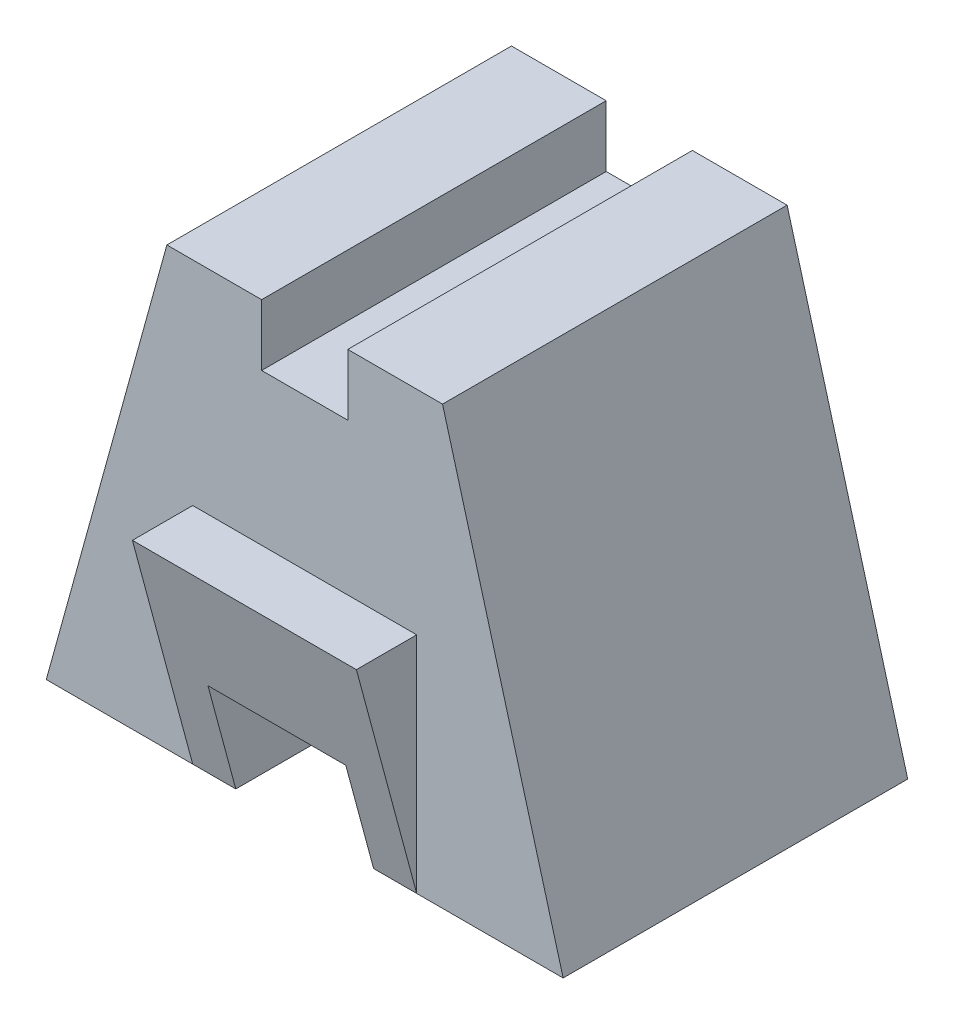
ISO-10303-21;
HEADER;
FILE_DESCRIPTION(('STEP AP214'),'2;1');
FILE_NAME('part.step','',(''),(''),'','','');
FILE_SCHEMA(('AUTOMOTIVE_DESIGN { 1 0 10303 214 1 1 1 1 }'));
ENDSEC;
DATA;
#1=APPLICATION_CONTEXT('core data for automotive mechanical design processes');
#2=APPLICATION_PROTOCOL_DEFINITION('international standard','automotive_design',2000,#1);
#3=PRODUCT_CONTEXT('',#1,'mechanical');
#4=PRODUCT('Part','Part','',(#3));
#5=PRODUCT_RELATED_PRODUCT_CATEGORY('part','',(#4));
#6=PRODUCT_DEFINITION_FORMATION('','',#4);
#7=PRODUCT_DEFINITION_CONTEXT('part definition',#1,'design');
#8=PRODUCT_DEFINITION('design','',#6,#7);
#9=PRODUCT_DEFINITION_SHAPE('','',#8);
#10=(LENGTH_UNIT() NAMED_UNIT(*) SI_UNIT(.MILLI.,.METRE.));
#11=(NAMED_UNIT(*) PLANE_ANGLE_UNIT() SI_UNIT($,.RADIAN.));
#12=(NAMED_UNIT(*) SI_UNIT($,.STERADIAN.) SOLID_ANGLE_UNIT());
#13=UNCERTAINTY_MEASURE_WITH_UNIT(LENGTH_MEASURE(1.E-05),#10,'distance_accuracy_value','');
#14=(GEOMETRIC_REPRESENTATION_CONTEXT(3) GLOBAL_UNCERTAINTY_ASSIGNED_CONTEXT((#13)) GLOBAL_UNIT_ASSIGNED_CONTEXT((#10,
#11,#12)) REPRESENTATION_CONTEXT('',''));
#15=CARTESIAN_POINT('',(0.,0.,0.));
#16=DIRECTION('',(0.,0.,1.));
#17=DIRECTION('',(1.,0.,0.));
#18=AXIS2_PLACEMENT_3D('',#15,#16,#17);
#19=CARTESIAN_POINT('',(-150.,0.,100.));
#20=DIRECTION('',(0.963916727737605,-0.266203948106761,0.));
#21=DIRECTION('',(0.266203948106761,0.963916727737605,0.));
#22=AXIS2_PLACEMENT_3D('',#19,#20,#21);
#23=PLANE('',#22);
#24=DIRECTION('',(-0.196974968900407,-0.713240614269742,-0.672672793996312));
#25=VECTOR('',#24,1.);
#26=CARTESIAN_POINT('',(-150.,0.,-100.));
#27=LINE('',#26,#25);
#28=CARTESIAN_POINT('',(-120.717565708256,106.030840051137,0.));
#29=VERTEX_POINT('',#28);
#30=CARTESIAN_POINT('',(-150.,0.,-100.));
#31=VERTEX_POINT('',#30);
#32=EDGE_CURVE('E163',#29,#31,#27,.T.);
#33=ORIENTED_EDGE('',*,*,#32,.F.);
#34=DIRECTION('',(0.196974968900407,0.713240614269742,-0.672672793996312));
#35=VECTOR('',#34,1.);
#36=CARTESIAN_POINT('',(-120.717565708256,106.030840051137,0.));
#37=LINE('',#36,#35);
#38=CARTESIAN_POINT('',(-150.,0.,100.));
#39=VERTEX_POINT('',#38);
#40=EDGE_CURVE('E175',#39,#29,#37,.T.);
#41=ORIENTED_EDGE('',*,*,#40,.F.);
#42=DIRECTION('',(-0.266203948106761,-0.963916727737605,0.));
#43=VECTOR('',#42,1.);
#44=CARTESIAN_POINT('',(-150.,0.,100.));
#45=LINE('',#44,#43);
#46=CARTESIAN_POINT('',(-80.,253.467957261745,100.));
#47=VERTEX_POINT('',#46);
#48=EDGE_CURVE('E229',#47,#39,#45,.T.);
#49=ORIENTED_EDGE('',*,*,#48,.F.);
#50=DIRECTION('',(0.,0.,-1.));
#51=VECTOR('',#50,1.);
#52=CARTESIAN_POINT('',(-80.,253.467957261745,100.));
#53=LINE('',#52,#51);
#54=CARTESIAN_POINT('',(-80.,253.467957261745,-100.));
#55=VERTEX_POINT('',#54);
#56=EDGE_CURVE('E275',#47,#55,#53,.T.);
#57=ORIENTED_EDGE('',*,*,#56,.T.);
#58=DIRECTION('',(-0.266203948106761,-0.963916727737605,0.));
#59=VECTOR('',#58,1.);
#60=CARTESIAN_POINT('',(-150.,0.,-100.));
#61=LINE('',#60,#59);
#62=EDGE_CURVE('E248',#55,#31,#61,.T.);
#63=ORIENTED_EDGE('',*,*,#62,.T.);
#64=EDGE_LOOP('',(#33,#41,#49,#57,#63));
#65=FACE_BOUND('',#64,.T.);
#66=ADVANCED_FACE('F39',(#65),#23,.F.);
#67=CARTESIAN_POINT('',(0.,0.,100.));
#68=DIRECTION('',(0.,0.,-1.));
#69=DIRECTION('',(-1.,0.,0.));
#70=AXIS2_PLACEMENT_3D('',#67,#68,#69);
#71=PLANE('',#70);
#72=DIRECTION('',(0.,-1.,0.));
#73=VECTOR('',#72,1.);
#74=CARTESIAN_POINT('',(-65.,130.,100.));
#75=LINE('',#74,#73);
#76=CARTESIAN_POINT('',(-65.,130.,100.));
#77=VERTEX_POINT('',#76);
#78=CARTESIAN_POINT('',(-65.,0.,100.));
#79=VERTEX_POINT('',#78);
#80=EDGE_CURVE('E61',#77,#79,#75,.T.);
#81=ORIENTED_EDGE('',*,*,#80,.F.);
#82=DIRECTION('',(-1.,0.,0.));
#83=VECTOR('',#82,1.);
#84=CARTESIAN_POINT('',(65.,130.,100.));
#85=LINE('',#84,#83);
#86=CARTESIAN_POINT('',(65.,130.,100.));
#87=VERTEX_POINT('',#86);
#88=EDGE_CURVE('E204',#87,#77,#85,.T.);
#89=ORIENTED_EDGE('',*,*,#88,.F.);
#90=DIRECTION('',(0.,1.,0.));
#91=VECTOR('',#90,1.);
#92=CARTESIAN_POINT('',(65.,0.,100.));
#93=LINE('',#92,#91);
#94=CARTESIAN_POINT('',(65.,0.,100.));
#95=VERTEX_POINT('',#94);
#96=EDGE_CURVE('E196',#95,#87,#93,.T.);
#97=ORIENTED_EDGE('',*,*,#96,.F.);
#98=DIRECTION('',(1.,0.,0.));
#99=VECTOR('',#98,1.);
#100=CARTESIAN_POINT('',(150.,0.,100.));
#101=LINE('',#100,#99);
#102=CARTESIAN_POINT('',(150.,0.,100.));
#103=VERTEX_POINT('',#102);
#104=EDGE_CURVE('E213',#95,#103,#101,.T.);
#105=ORIENTED_EDGE('',*,*,#104,.T.);
#106=DIRECTION('',(-0.266203948106761,0.963916727737605,0.));
#107=VECTOR('',#106,1.);
#108=CARTESIAN_POINT('',(80.,253.467957261745,100.));
#109=LINE('',#108,#107);
#110=CARTESIAN_POINT('',(80.,253.467957261745,100.));
#111=VERTEX_POINT('',#110);
#112=EDGE_CURVE('E214',#103,#111,#109,.T.);
#113=ORIENTED_EDGE('',*,*,#112,.T.);
#114=DIRECTION('',(-1.,0.,0.));
#115=VECTOR('',#114,1.);
#116=CARTESIAN_POINT('',(25.,253.467957261745,100.));
#117=LINE('',#116,#115);
#118=CARTESIAN_POINT('',(25.,253.467957261745,100.));
#119=VERTEX_POINT('',#118);
#120=EDGE_CURVE('E217',#111,#119,#117,.T.);
#121=ORIENTED_EDGE('',*,*,#120,.T.);
#122=DIRECTION('',(0.,-1.,0.));
#123=VECTOR('',#122,1.);
#124=CARTESIAN_POINT('',(25.,217.876631194631,100.));
#125=LINE('',#124,#123);
#126=CARTESIAN_POINT('',(25.,217.876631194631,100.));
#127=VERTEX_POINT('',#126);
#128=EDGE_CURVE('E219',#119,#127,#125,.T.);
#129=ORIENTED_EDGE('',*,*,#128,.T.);
#130=DIRECTION('',(-1.,0.,0.));
#131=VECTOR('',#130,1.);
#132=CARTESIAN_POINT('',(-25.,217.876631194631,100.));
#133=LINE('',#132,#131);
#134=CARTESIAN_POINT('',(-25.,217.876631194631,100.));
#135=VERTEX_POINT('',#134);
#136=EDGE_CURVE('E225',#127,#135,#133,.T.);
#137=ORIENTED_EDGE('',*,*,#136,.T.);
#138=DIRECTION('',(0.,1.,0.));
#139=VECTOR('',#138,1.);
#140=CARTESIAN_POINT('',(-25.,253.467957261745,100.));
#141=LINE('',#140,#139);
#142=CARTESIAN_POINT('',(-25.,253.467957261745,100.));
#143=VERTEX_POINT('',#142);
#144=EDGE_CURVE('E221',#135,#143,#141,.T.);
#145=ORIENTED_EDGE('',*,*,#144,.T.);
#146=DIRECTION('',(-1.,0.,0.));
#147=VECTOR('',#146,1.);
#148=CARTESIAN_POINT('',(-80.,253.467957261745,100.));
#149=LINE('',#148,#147);
#150=EDGE_CURVE('E226',#143,#47,#149,.T.);
#151=ORIENTED_EDGE('',*,*,#150,.T.);
#152=ORIENTED_EDGE('',*,*,#48,.T.);
#153=DIRECTION('',(1.,0.,0.));
#154=VECTOR('',#153,1.);
#155=CARTESIAN_POINT('',(-40.,0.,100.));
#156=LINE('',#155,#154);
#157=EDGE_CURVE('E232',#39,#79,#156,.T.);
#158=ORIENTED_EDGE('',*,*,#157,.T.);
#159=EDGE_LOOP('',(#81,#89,#97,#105,#113,#121,#129,#137,#145,#151,#152,#158));
#160=FACE_BOUND('',#159,.T.);
#161=ADVANCED_FACE('F316',(#160),#71,.F.);
#162=CARTESIAN_POINT('',(150.,0.,100.));
#163=DIRECTION('',(0.,1.,0.));
#164=DIRECTION('',(-1.,0.,0.));
#165=AXIS2_PLACEMENT_3D('',#162,#163,#164);
#166=PLANE('',#165);
#167=ORIENTED_EDGE('',*,*,#104,.F.);
#168=DIRECTION('',(-1.,0.,0.));
#169=VECTOR('',#168,1.);
#170=CARTESIAN_POINT('',(150.,0.,100.));
#171=LINE('',#170,#169);
#172=CARTESIAN_POINT('',(40.,0.,100.));
#173=VERTEX_POINT('',#172);
#174=EDGE_CURVE('E183',#95,#173,#171,.T.);
#175=ORIENTED_EDGE('',*,*,#174,.T.);
#176=DIRECTION('',(0.,0.,-1.));
#177=VECTOR('',#176,1.);
#178=CARTESIAN_POINT('',(40.,0.,100.));
#179=LINE('',#178,#177);
#180=CARTESIAN_POINT('',(40.,0.,-100.));
#181=VERTEX_POINT('',#180);
#182=EDGE_CURVE('E233',#173,#181,#179,.T.);
#183=ORIENTED_EDGE('',*,*,#182,.T.);
#184=DIRECTION('',(1.,0.,0.));
#185=VECTOR('',#184,1.);
#186=CARTESIAN_POINT('',(150.,0.,-100.));
#187=LINE('',#186,#185);
#188=CARTESIAN_POINT('',(150.,0.,-100.));
#189=VERTEX_POINT('',#188);
#190=EDGE_CURVE('E215',#181,#189,#187,.T.);
#191=ORIENTED_EDGE('',*,*,#190,.T.);
#192=DIRECTION('',(0.,0.,-1.));
#193=VECTOR('',#192,1.);
#194=CARTESIAN_POINT('',(150.,0.,100.));
#195=LINE('',#194,#193);
#196=EDGE_CURVE('E50',#103,#189,#195,.T.);
#197=ORIENTED_EDGE('',*,*,#196,.F.);
#198=EDGE_LOOP('',(#167,#175,#183,#191,#197));
#199=FACE_BOUND('',#198,.T.);
#200=ADVANCED_FACE('F41',(#199),#166,.F.);
#201=CARTESIAN_POINT('',(80.,253.467957261745,100.));
#202=DIRECTION('',(-0.963916727737605,-0.266203948106761,0.));
#203=DIRECTION('',(0.266203948106761,-0.963916727737605,0.));
#204=AXIS2_PLACEMENT_3D('',#201,#202,#203);
#205=PLANE('',#204);
#206=DIRECTION('',(-0.266203948106761,0.963916727737605,0.));
#207=VECTOR('',#206,1.);
#208=CARTESIAN_POINT('',(80.,253.467957261745,-100.));
#209=LINE('',#208,#207);
#210=CARTESIAN_POINT('',(80.,253.467957261745,-100.));
#211=VERTEX_POINT('',#210);
#212=EDGE_CURVE('E237',#189,#211,#209,.T.);
#213=ORIENTED_EDGE('',*,*,#212,.T.);
#214=DIRECTION('',(0.,0.,-1.));
#215=VECTOR('',#214,1.);
#216=CARTESIAN_POINT('',(80.,253.467957261745,100.));
#217=LINE('',#216,#215);
#218=EDGE_CURVE('E290',#111,#211,#217,.T.);
#219=ORIENTED_EDGE('',*,*,#218,.F.);
#220=ORIENTED_EDGE('',*,*,#112,.F.);
#221=ORIENTED_EDGE('',*,*,#196,.T.);
#222=EDGE_LOOP('',(#213,#219,#220,#221));
#223=FACE_BOUND('',#222,.T.);
#224=ADVANCED_FACE('F291',(#223),#205,.F.);
#225=CARTESIAN_POINT('',(25.,253.467957261745,100.));
#226=DIRECTION('',(0.,-1.,0.));
#227=DIRECTION('',(0.,0.,-1.));
#228=AXIS2_PLACEMENT_3D('',#225,#226,#227);
#229=PLANE('',#228);
#230=DIRECTION('',(-1.,0.,0.));
#231=VECTOR('',#230,1.);
#232=CARTESIAN_POINT('',(25.,253.467957261745,-100.));
#233=LINE('',#232,#231);
#234=CARTESIAN_POINT('',(25.,253.467957261745,-100.));
#235=VERTEX_POINT('',#234);
#236=EDGE_CURVE('E236',#211,#235,#233,.T.);
#237=ORIENTED_EDGE('',*,*,#236,.T.);
#238=DIRECTION('',(0.,0.,-1.));
#239=VECTOR('',#238,1.);
#240=CARTESIAN_POINT('',(25.,253.467957261745,100.));
#241=LINE('',#240,#239);
#242=EDGE_CURVE('E283',#119,#235,#241,.T.);
#243=ORIENTED_EDGE('',*,*,#242,.F.);
#244=ORIENTED_EDGE('',*,*,#120,.F.);
#245=ORIENTED_EDGE('',*,*,#218,.T.);
#246=EDGE_LOOP('',(#237,#243,#244,#245));
#247=FACE_BOUND('',#246,.T.);
#248=ADVANCED_FACE('F310',(#247),#229,.F.);
#249=CARTESIAN_POINT('',(25.,217.876631194631,100.));
#250=DIRECTION('',(1.,0.,0.));
#251=DIRECTION('',(0.,0.,-1.));
#252=AXIS2_PLACEMENT_3D('',#249,#250,#251);
#253=PLANE('',#252);
#254=DIRECTION('',(0.,-1.,0.));
#255=VECTOR('',#254,1.);
#256=CARTESIAN_POINT('',(25.,217.876631194631,-100.));
#257=LINE('',#256,#255);
#258=CARTESIAN_POINT('',(25.,217.876631194631,-100.));
#259=VERTEX_POINT('',#258);
#260=EDGE_CURVE('E238',#235,#259,#257,.T.);
#261=ORIENTED_EDGE('',*,*,#260,.T.);
#262=DIRECTION('',(0.,0.,-1.));
#263=VECTOR('',#262,1.);
#264=CARTESIAN_POINT('',(25.,217.876631194631,100.));
#265=LINE('',#264,#263);
#266=EDGE_CURVE('E281',#127,#259,#265,.T.);
#267=ORIENTED_EDGE('',*,*,#266,.F.);
#268=ORIENTED_EDGE('',*,*,#128,.F.);
#269=ORIENTED_EDGE('',*,*,#242,.T.);
#270=EDGE_LOOP('',(#261,#267,#268,#269));
#271=FACE_BOUND('',#270,.T.);
#272=ADVANCED_FACE('F311',(#271),#253,.F.);
#273=CARTESIAN_POINT('',(-25.,217.876631194631,100.));
#274=DIRECTION('',(0.,-1.,0.));
#275=DIRECTION('',(0.,0.,-1.));
#276=AXIS2_PLACEMENT_3D('',#273,#274,#275);
#277=PLANE('',#276);
#278=DIRECTION('',(-1.,0.,0.));
#279=VECTOR('',#278,1.);
#280=CARTESIAN_POINT('',(-25.,217.876631194631,-100.));
#281=LINE('',#280,#279);
#282=CARTESIAN_POINT('',(-25.,217.876631194631,-100.));
#283=VERTEX_POINT('',#282);
#284=EDGE_CURVE('E242',#259,#283,#281,.T.);
#285=ORIENTED_EDGE('',*,*,#284,.T.);
#286=DIRECTION('',(0.,0.,-1.));
#287=VECTOR('',#286,1.);
#288=CARTESIAN_POINT('',(-25.,217.876631194631,100.));
#289=LINE('',#288,#287);
#290=EDGE_CURVE('E279',#135,#283,#289,.T.);
#291=ORIENTED_EDGE('',*,*,#290,.F.);
#292=ORIENTED_EDGE('',*,*,#136,.F.);
#293=ORIENTED_EDGE('',*,*,#266,.T.);
#294=EDGE_LOOP('',(#285,#291,#292,#293));
#295=FACE_BOUND('',#294,.T.);
#296=ADVANCED_FACE('F352',(#295),#277,.F.);
#297=CARTESIAN_POINT('',(-25.,253.467957261745,100.));
#298=DIRECTION('',(-1.,0.,0.));
#299=DIRECTION('',(0.,-1.,0.));
#300=AXIS2_PLACEMENT_3D('',#297,#298,#299);
#301=PLANE('',#300);
#302=DIRECTION('',(0.,1.,0.));
#303=VECTOR('',#302,1.);
#304=CARTESIAN_POINT('',(-25.,253.467957261745,-100.));
#305=LINE('',#304,#303);
#306=CARTESIAN_POINT('',(-25.,253.467957261745,-100.));
#307=VERTEX_POINT('',#306);
#308=EDGE_CURVE('E243',#283,#307,#305,.T.);
#309=ORIENTED_EDGE('',*,*,#308,.T.);
#310=DIRECTION('',(0.,0.,-1.));
#311=VECTOR('',#310,1.);
#312=CARTESIAN_POINT('',(-25.,253.467957261745,100.));
#313=LINE('',#312,#311);
#314=EDGE_CURVE('E274',#143,#307,#313,.T.);
#315=ORIENTED_EDGE('',*,*,#314,.F.);
#316=ORIENTED_EDGE('',*,*,#144,.F.);
#317=ORIENTED_EDGE('',*,*,#290,.T.);
#318=EDGE_LOOP('',(#309,#315,#316,#317));
#319=FACE_BOUND('',#318,.T.);
#320=ADVANCED_FACE('F348',(#319),#301,.F.);
#321=CARTESIAN_POINT('',(-80.,253.467957261745,100.));
#322=DIRECTION('',(0.,-1.,0.));
#323=DIRECTION('',(0.,0.,-1.));
#324=AXIS2_PLACEMENT_3D('',#321,#322,#323);
#325=PLANE('',#324);
#326=DIRECTION('',(-1.,0.,0.));
#327=VECTOR('',#326,1.);
#328=CARTESIAN_POINT('',(-80.,253.467957261745,-100.));
#329=LINE('',#328,#327);
#330=EDGE_CURVE('E247',#307,#55,#329,.T.);
#331=ORIENTED_EDGE('',*,*,#330,.T.);
#332=ORIENTED_EDGE('',*,*,#56,.F.);
#333=ORIENTED_EDGE('',*,*,#150,.F.);
#334=ORIENTED_EDGE('',*,*,#314,.T.);
#335=EDGE_LOOP('',(#331,#332,#333,#334));
#336=FACE_BOUND('',#335,.T.);
#337=ADVANCED_FACE('F341',(#336),#325,.F.);
#338=CARTESIAN_POINT('',(-40.,0.,100.));
#339=DIRECTION('',(0.,1.,0.));
#340=DIRECTION('',(-1.,0.,0.));
#341=AXIS2_PLACEMENT_3D('',#338,#339,#340);
#342=PLANE('',#341);
#343=DIRECTION('',(0.,0.,-1.));
#344=VECTOR('',#343,1.);
#345=CARTESIAN_POINT('',(-40.,0.,100.));
#346=LINE('',#345,#344);
#347=CARTESIAN_POINT('',(-40.,0.,100.));
#348=VERTEX_POINT('',#347);
#349=CARTESIAN_POINT('',(-40.,0.,-100.));
#350=VERTEX_POINT('',#349);
#351=EDGE_CURVE('E270',#348,#350,#346,.T.);
#352=ORIENTED_EDGE('',*,*,#351,.F.);
#353=EDGE_CURVE('E178',#348,#79,#171,.T.);
#354=ORIENTED_EDGE('',*,*,#353,.T.);
#355=ORIENTED_EDGE('',*,*,#157,.F.);
#356=DIRECTION('',(0.,0.,-1.));
#357=VECTOR('',#356,1.);
#358=CARTESIAN_POINT('',(-150.,0.,100.));
#359=LINE('',#358,#357);
#360=EDGE_CURVE('E267',#39,#31,#359,.T.);
#361=ORIENTED_EDGE('',*,*,#360,.T.);
#362=DIRECTION('',(1.,0.,0.));
#363=VECTOR('',#362,1.);
#364=CARTESIAN_POINT('',(-40.,0.,-100.));
#365=LINE('',#364,#363);
#366=EDGE_CURVE('E253',#31,#350,#365,.T.);
#367=ORIENTED_EDGE('',*,*,#366,.T.);
#368=EDGE_LOOP('',(#352,#354,#355,#361,#367));
#369=FACE_BOUND('',#368,.T.);
#370=ADVANCED_FACE('F334',(#369),#342,.F.);
#371=CARTESIAN_POINT('',(-40.,60.,100.));
#372=DIRECTION('',(-1.,0.,0.));
#373=DIRECTION('',(0.,0.,1.));
#374=AXIS2_PLACEMENT_3D('',#371,#372,#373);
#375=PLANE('',#374);
#376=DIRECTION('',(0.,0.,-1.));
#377=VECTOR('',#376,1.);
#378=CARTESIAN_POINT('',(-40.,60.,100.));
#379=LINE('',#378,#377);
#380=CARTESIAN_POINT('',(-40.,60.,116.153846153846));
#381=VERTEX_POINT('',#380);
#382=CARTESIAN_POINT('',(-40.,60.,-100.));
#383=VERTEX_POINT('',#382);
#384=EDGE_CURVE('E264',#381,#383,#379,.T.);
#385=ORIENTED_EDGE('',*,*,#384,.F.);
#386=DIRECTION('',(0.,-0.96561575852067,-0.259973473447873));
#387=VECTOR('',#386,1.);
#388=CARTESIAN_POINT('',(-40.,55.9448275862069,115.062068965517));
#389=LINE('',#388,#387);
#390=EDGE_CURVE('E191',#381,#348,#389,.T.);
#391=ORIENTED_EDGE('',*,*,#390,.T.);
#392=ORIENTED_EDGE('',*,*,#351,.T.);
#393=DIRECTION('',(0.,1.,0.));
#394=VECTOR('',#393,1.);
#395=CARTESIAN_POINT('',(-40.,60.,-100.));
#396=LINE('',#395,#394);
#397=EDGE_CURVE('E255',#350,#383,#396,.T.);
#398=ORIENTED_EDGE('',*,*,#397,.T.);
#399=EDGE_LOOP('',(#385,#391,#392,#398));
#400=FACE_BOUND('',#399,.T.);
#401=ADVANCED_FACE('F329',(#400),#375,.F.);
#402=CARTESIAN_POINT('',(40.,60.,100.));
#403=DIRECTION('',(0.,1.,0.));
#404=DIRECTION('',(-1.,0.,0.));
#405=AXIS2_PLACEMENT_3D('',#402,#403,#404);
#406=PLANE('',#405);
#407=DIRECTION('',(0.,0.,-1.));
#408=VECTOR('',#407,1.);
#409=CARTESIAN_POINT('',(40.,60.,100.));
#410=LINE('',#409,#408);
#411=CARTESIAN_POINT('',(40.,60.,116.153846153846));
#412=VERTEX_POINT('',#411);
#413=CARTESIAN_POINT('',(40.,60.,-100.));
#414=VERTEX_POINT('',#413);
#415=EDGE_CURVE('E263',#412,#414,#410,.T.);
#416=ORIENTED_EDGE('',*,*,#415,.F.);
#417=DIRECTION('',(-1.,0.,0.));
#418=VECTOR('',#417,1.);
#419=CARTESIAN_POINT('',(40.,60.,116.153846153846));
#420=LINE('',#419,#418);
#421=EDGE_CURVE('E195',#412,#381,#420,.T.);
#422=ORIENTED_EDGE('',*,*,#421,.T.);
#423=ORIENTED_EDGE('',*,*,#384,.T.);
#424=DIRECTION('',(1.,0.,0.));
#425=VECTOR('',#424,1.);
#426=CARTESIAN_POINT('',(40.,60.,-100.));
#427=LINE('',#426,#425);
#428=EDGE_CURVE('E260',#383,#414,#427,.T.);
#429=ORIENTED_EDGE('',*,*,#428,.T.);
#430=EDGE_LOOP('',(#416,#422,#423,#429));
#431=FACE_BOUND('',#430,.T.);
#432=ADVANCED_FACE('F322',(#431),#406,.F.);
#433=CARTESIAN_POINT('',(40.,0.,100.));
#434=DIRECTION('',(1.,0.,0.));
#435=DIRECTION('',(0.,0.,-1.));
#436=AXIS2_PLACEMENT_3D('',#433,#434,#435);
#437=PLANE('',#436);
#438=ORIENTED_EDGE('',*,*,#182,.F.);
#439=DIRECTION('',(0.,0.96561575852067,0.259973473447873));
#440=VECTOR('',#439,1.);
#441=CARTESIAN_POINT('',(40.,0.,100.));
#442=LINE('',#441,#440);
#443=EDGE_CURVE('E188',#173,#412,#442,.T.);
#444=ORIENTED_EDGE('',*,*,#443,.T.);
#445=ORIENTED_EDGE('',*,*,#415,.T.);
#446=DIRECTION('',(0.,-1.,0.));
#447=VECTOR('',#446,1.);
#448=CARTESIAN_POINT('',(40.,0.,-100.));
#449=LINE('',#448,#447);
#450=EDGE_CURVE('E216',#414,#181,#449,.T.);
#451=ORIENTED_EDGE('',*,*,#450,.T.);
#452=EDGE_LOOP('',(#438,#444,#445,#451));
#453=FACE_BOUND('',#452,.T.);
#454=ADVANCED_FACE('F321',(#453),#437,.F.);
#455=CARTESIAN_POINT('',(0.,0.,-100.));
#456=DIRECTION('',(0.,0.,-1.));
#457=DIRECTION('',(-1.,0.,0.));
#458=AXIS2_PLACEMENT_3D('',#455,#456,#457);
#459=PLANE('',#458);
#460=ORIENTED_EDGE('',*,*,#190,.F.);
#461=ORIENTED_EDGE('',*,*,#450,.F.);
#462=ORIENTED_EDGE('',*,*,#428,.F.);
#463=ORIENTED_EDGE('',*,*,#397,.F.);
#464=ORIENTED_EDGE('',*,*,#366,.F.);
#465=ORIENTED_EDGE('',*,*,#62,.F.);
#466=ORIENTED_EDGE('',*,*,#330,.F.);
#467=ORIENTED_EDGE('',*,*,#308,.F.);
#468=ORIENTED_EDGE('',*,*,#284,.F.);
#469=ORIENTED_EDGE('',*,*,#260,.F.);
#470=ORIENTED_EDGE('',*,*,#236,.F.);
#471=ORIENTED_EDGE('',*,*,#212,.F.);
#472=EDGE_LOOP('',(#460,#461,#462,#463,#464,#465,#466,#467,#468,#469,#470,#471));
#473=FACE_BOUND('',#472,.T.);
#474=ADVANCED_FACE('F305',(#473),#459,.T.);
#475=CARTESIAN_POINT('',(65.,0.,135.));
#476=DIRECTION('',(-1.,0.,0.));
#477=DIRECTION('',(0.,0.,1.));
#478=AXIS2_PLACEMENT_3D('',#475,#476,#477);
#479=PLANE('',#478);
#480=DIRECTION('',(0.,0.,-1.));
#481=VECTOR('',#480,1.);
#482=CARTESIAN_POINT('',(65.,130.,135.));
#483=LINE('',#482,#481);
#484=CARTESIAN_POINT('',(65.,130.,135.));
#485=VERTEX_POINT('',#484);
#486=EDGE_CURVE('E207',#485,#87,#483,.T.);
#487=ORIENTED_EDGE('',*,*,#486,.F.);
#488=DIRECTION('',(0.,-0.96561575852067,-0.259973473447873));
#489=VECTOR('',#488,1.);
#490=CARTESIAN_POINT('',(65.,8.7862068965517,102.365517241379));
#491=LINE('',#490,#489);
#492=EDGE_CURVE('E186',#485,#95,#491,.T.);
#493=ORIENTED_EDGE('',*,*,#492,.T.);
#494=ORIENTED_EDGE('',*,*,#96,.T.);
#495=EDGE_LOOP('',(#487,#493,#494));
#496=FACE_BOUND('',#495,.T.);
#497=ADVANCED_FACE('F387',(#496),#479,.F.);
#498=CARTESIAN_POINT('',(65.,130.,135.));
#499=DIRECTION('',(0.,-1.,0.));
#500=DIRECTION('',(1.,0.,0.));
#501=AXIS2_PLACEMENT_3D('',#498,#499,#500);
#502=PLANE('',#501);
#503=ORIENTED_EDGE('',*,*,#88,.T.);
#504=DIRECTION('',(0.,0.,-1.));
#505=VECTOR('',#504,1.);
#506=CARTESIAN_POINT('',(-65.,130.,135.));
#507=LINE('',#506,#505);
#508=CARTESIAN_POINT('',(-65.,130.,135.));
#509=VERTEX_POINT('',#508);
#510=EDGE_CURVE('E203',#509,#77,#507,.T.);
#511=ORIENTED_EDGE('',*,*,#510,.F.);
#512=DIRECTION('',(-1.,0.,0.));
#513=VECTOR('',#512,1.);
#514=CARTESIAN_POINT('',(65.,130.,135.));
#515=LINE('',#514,#513);
#516=EDGE_CURVE('E200',#485,#509,#515,.T.);
#517=ORIENTED_EDGE('',*,*,#516,.F.);
#518=ORIENTED_EDGE('',*,*,#486,.T.);
#519=EDGE_LOOP('',(#503,#511,#517,#518));
#520=FACE_BOUND('',#519,.T.);
#521=ADVANCED_FACE('F388',(#520),#502,.F.);
#522=CARTESIAN_POINT('',(-65.,130.,135.));
#523=DIRECTION('',(1.,0.,0.));
#524=DIRECTION('',(0.,0.,-1.));
#525=AXIS2_PLACEMENT_3D('',#522,#523,#524);
#526=PLANE('',#525);
#527=ORIENTED_EDGE('',*,*,#80,.T.);
#528=DIRECTION('',(0.,-0.965615758520669,-0.259973473447873));
#529=VECTOR('',#528,1.);
#530=CARTESIAN_POINT('',(-65.,0.,100.));
#531=LINE('',#530,#529);
#532=EDGE_CURVE('E177',#509,#79,#531,.T.);
#533=ORIENTED_EDGE('',*,*,#532,.F.);
#534=ORIENTED_EDGE('',*,*,#510,.T.);
#535=EDGE_LOOP('',(#527,#533,#534));
#536=FACE_BOUND('',#535,.T.);
#537=ADVANCED_FACE('F393',(#536),#526,.F.);
#538=CARTESIAN_POINT('',(150.,0.,100.));
#539=DIRECTION('',(0.,0.259973473447873,-0.965615758520669));
#540=DIRECTION('',(0.,0.96561575852067,0.259973473447873));
#541=AXIS2_PLACEMENT_3D('',#538,#539,#540);
#542=PLANE('',#541);
#543=ORIENTED_EDGE('',*,*,#421,.F.);
#544=ORIENTED_EDGE('',*,*,#443,.F.);
#545=ORIENTED_EDGE('',*,*,#174,.F.);
#546=ORIENTED_EDGE('',*,*,#492,.F.);
#547=ORIENTED_EDGE('',*,*,#516,.T.);
#548=ORIENTED_EDGE('',*,*,#532,.T.);
#549=ORIENTED_EDGE('',*,*,#353,.F.);
#550=ORIENTED_EDGE('',*,*,#390,.F.);
#551=EDGE_LOOP('',(#543,#544,#545,#546,#547,#548,#549,#550));
#552=FACE_BOUND('',#551,.T.);
#553=ADVANCED_FACE('F398',(#552),#542,.F.);
#554=CARTESIAN_POINT('',(-183.737085470816,9.31713818373665,-100.));
#555=DIRECTION('',(0.266203948106761,0.963916727737605,0.));
#556=DIRECTION('',(-0.963916727737605,0.266203948106761,0.));
#557=AXIS2_PLACEMENT_3D('',#554,#555,#556);
#558=PLANE('',#557);
#559=DIRECTION('',(-0.15077735271579,0.0416400353091031,-0.987690385377662));
#560=VECTOR('',#559,1.);
#561=CARTESIAN_POINT('',(-180.609737297005,8.45346147078331,-100.513821755283));
#562=LINE('',#561,#560);
#563=CARTESIAN_POINT('',(-165.265649534306,4.21589963065007,0.));
#564=VERTEX_POINT('',#563);
#565=EDGE_CURVE('E166',#39,#564,#562,.T.);
#566=ORIENTED_EDGE('',*,*,#565,.T.);
#567=DIRECTION('',(0.15077735271579,-0.0416400353091031,-0.987690385377662));
#568=VECTOR('',#567,1.);
#569=CARTESIAN_POINT('',(-150.825468974988,0.227968966465804,-94.592637718212));
#570=LINE('',#569,#568);
#571=EDGE_CURVE('E53',#564,#31,#570,.T.);
#572=ORIENTED_EDGE('',*,*,#571,.T.);
#573=ORIENTED_EDGE('',*,*,#360,.F.);
#574=EDGE_LOOP('',(#566,#572,#573));
#575=FACE_BOUND('',#574,.T.);
#576=ADVANCED_FACE('F337',(#575),#558,.F.);
#577=CARTESIAN_POINT('',(-154.454651179072,115.347978234873,0.));
#578=DIRECTION('',(-0.179068153545825,-0.648400558427038,-0.739940073395944));
#579=DIRECTION('',(0.,0.752096455392655,-0.659053049295582));
#580=AXIS2_PLACEMENT_3D('',#577,#578,#579);
#581=PLANE('',#580);
#582=DIRECTION('',(0.963916727737605,-0.266203948106761,0.));
#583=VECTOR('',#582,1.);
#584=CARTESIAN_POINT('',(-154.454651179072,115.347978234873,0.));
#585=LINE('',#584,#583);
#586=CARTESIAN_POINT('',(-154.454651179072,115.347978234873,0.));
#587=VERTEX_POINT('',#586);
#588=EDGE_CURVE('E162',#587,#29,#585,.T.);
#589=ORIENTED_EDGE('',*,*,#588,.F.);
#590=DIRECTION('',(-0.0291677464523161,0.755264654334308,-0.654770604471651));
#591=VECTOR('',#590,1.);
#592=CARTESIAN_POINT('',(-150.,0.,100.));
#593=LINE('',#592,#591);
#594=EDGE_CURVE('E170',#39,#587,#593,.T.);
#595=ORIENTED_EDGE('',*,*,#594,.F.);
#596=ORIENTED_EDGE('',*,*,#40,.T.);
#597=EDGE_LOOP('',(#589,#595,#596));
#598=FACE_BOUND('',#597,.T.);
#599=ADVANCED_FACE('F173',(#598),#581,.F.);
#600=CARTESIAN_POINT('',(-183.737085470816,9.31713818373665,-100.));
#601=DIRECTION('',(-0.179068153545825,-0.648400558427038,0.739940073395944));
#602=DIRECTION('',(0.,-0.752096455392655,-0.659053049295582));
#603=AXIS2_PLACEMENT_3D('',#600,#601,#602);
#604=PLANE('',#603);
#605=ORIENTED_EDGE('',*,*,#32,.T.);
#606=DIRECTION('',(0.0291677464523161,-0.755264654334308,-0.654770604471651));
#607=VECTOR('',#606,1.);
#608=CARTESIAN_POINT('',(-150.,0.,-100.));
#609=LINE('',#608,#607);
#610=EDGE_CURVE('E152',#587,#31,#609,.T.);
#611=ORIENTED_EDGE('',*,*,#610,.F.);
#612=ORIENTED_EDGE('',*,*,#588,.T.);
#613=EDGE_LOOP('',(#605,#611,#612));
#614=FACE_BOUND('',#613,.T.);
#615=ADVANCED_FACE('F161',(#614),#604,.F.);
#616=CARTESIAN_POINT('',(-177.581733797907,-99.8726531927529,-13.9724162375301));
#617=DIRECTION('',(0.983404209342518,-0.095666178688101,-0.15415623017781));
#618=DIRECTION('',(-0.154866529695688,0.,-0.987935401724229));
#619=AXIS2_PLACEMENT_3D('',#616,#617,#618);
#620=PLANE('',#619);
#621=ORIENTED_EDGE('',*,*,#594,.T.);
#622=DIRECTION('',(-0.0968235605629955,-0.9953015613973,0.));
#623=VECTOR('',#622,1.);
#624=CARTESIAN_POINT('',(-175.411982764338,-100.083727935076,0.));
#625=LINE('',#624,#623);
#626=EDGE_CURVE('E11',#587,#564,#625,.T.);
#627=ORIENTED_EDGE('',*,*,#626,.T.);
#628=ORIENTED_EDGE('',*,*,#565,.F.);
#629=EDGE_LOOP('',(#621,#627,#628));
#630=FACE_BOUND('',#629,.T.);
#631=ADVANCED_FACE('F169',(#630),#620,.F.);
#632=CARTESIAN_POINT('',(-182.116428556734,-116.292650583117,32.710546419992));
#633=DIRECTION('',(0.983404209342518,-0.0956661786881009,0.15415623017781));
#634=DIRECTION('',(0.154866529695688,0.,-0.987935401724229));
#635=AXIS2_PLACEMENT_3D('',#632,#633,#634);
#636=PLANE('',#635);
#637=ORIENTED_EDGE('',*,*,#626,.F.);
#638=ORIENTED_EDGE('',*,*,#610,.T.);
#639=ORIENTED_EDGE('',*,*,#571,.F.);
#640=EDGE_LOOP('',(#637,#638,#639));
#641=FACE_BOUND('',#640,.T.);
#642=ADVANCED_FACE('F153',(#641),#636,.F.);
#643=CLOSED_SHELL('',(#66,#161,#200,#224,#248,#272,#296,#320,#337,#370,#401,#432,#454,#474,#497,
#521,#537,#553,#576,#599,#615,#631,#642));
#644=MANIFOLD_SOLID_BREP('B2',#643);
#645=ADVANCED_BREP_SHAPE_REPRESENTATION('',(#18,#644),#14);
#646=SHAPE_DEFINITION_REPRESENTATION(#9,#645);
ENDSEC;
END-ISO-10303-21;
